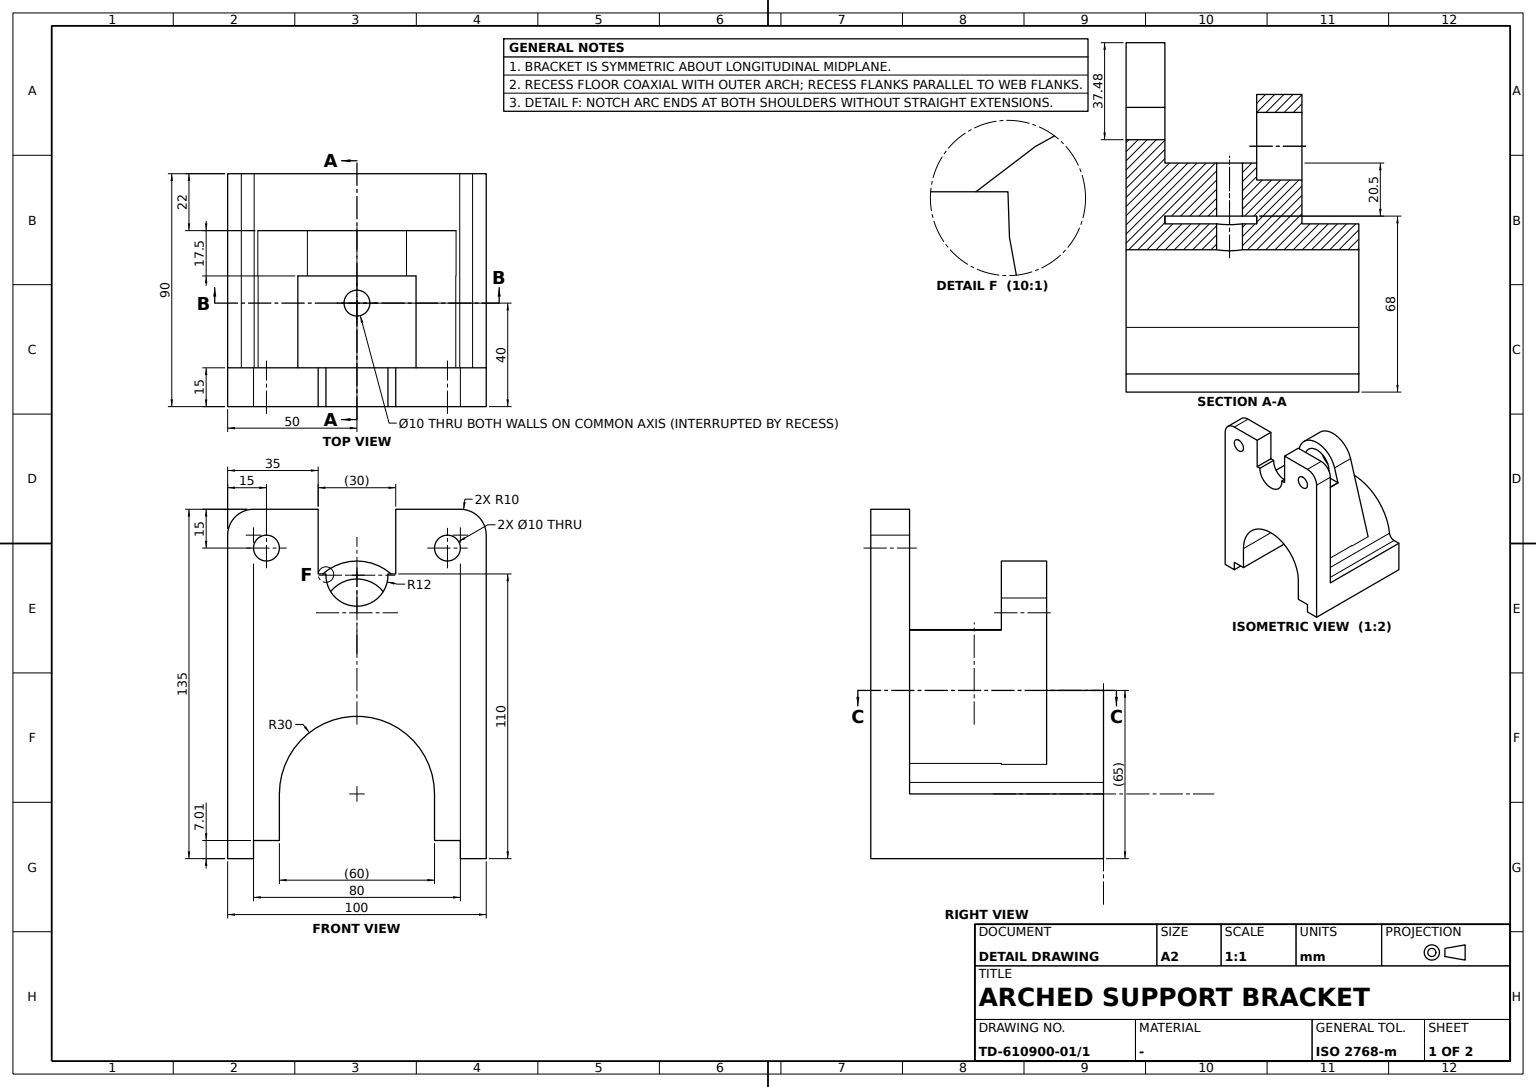
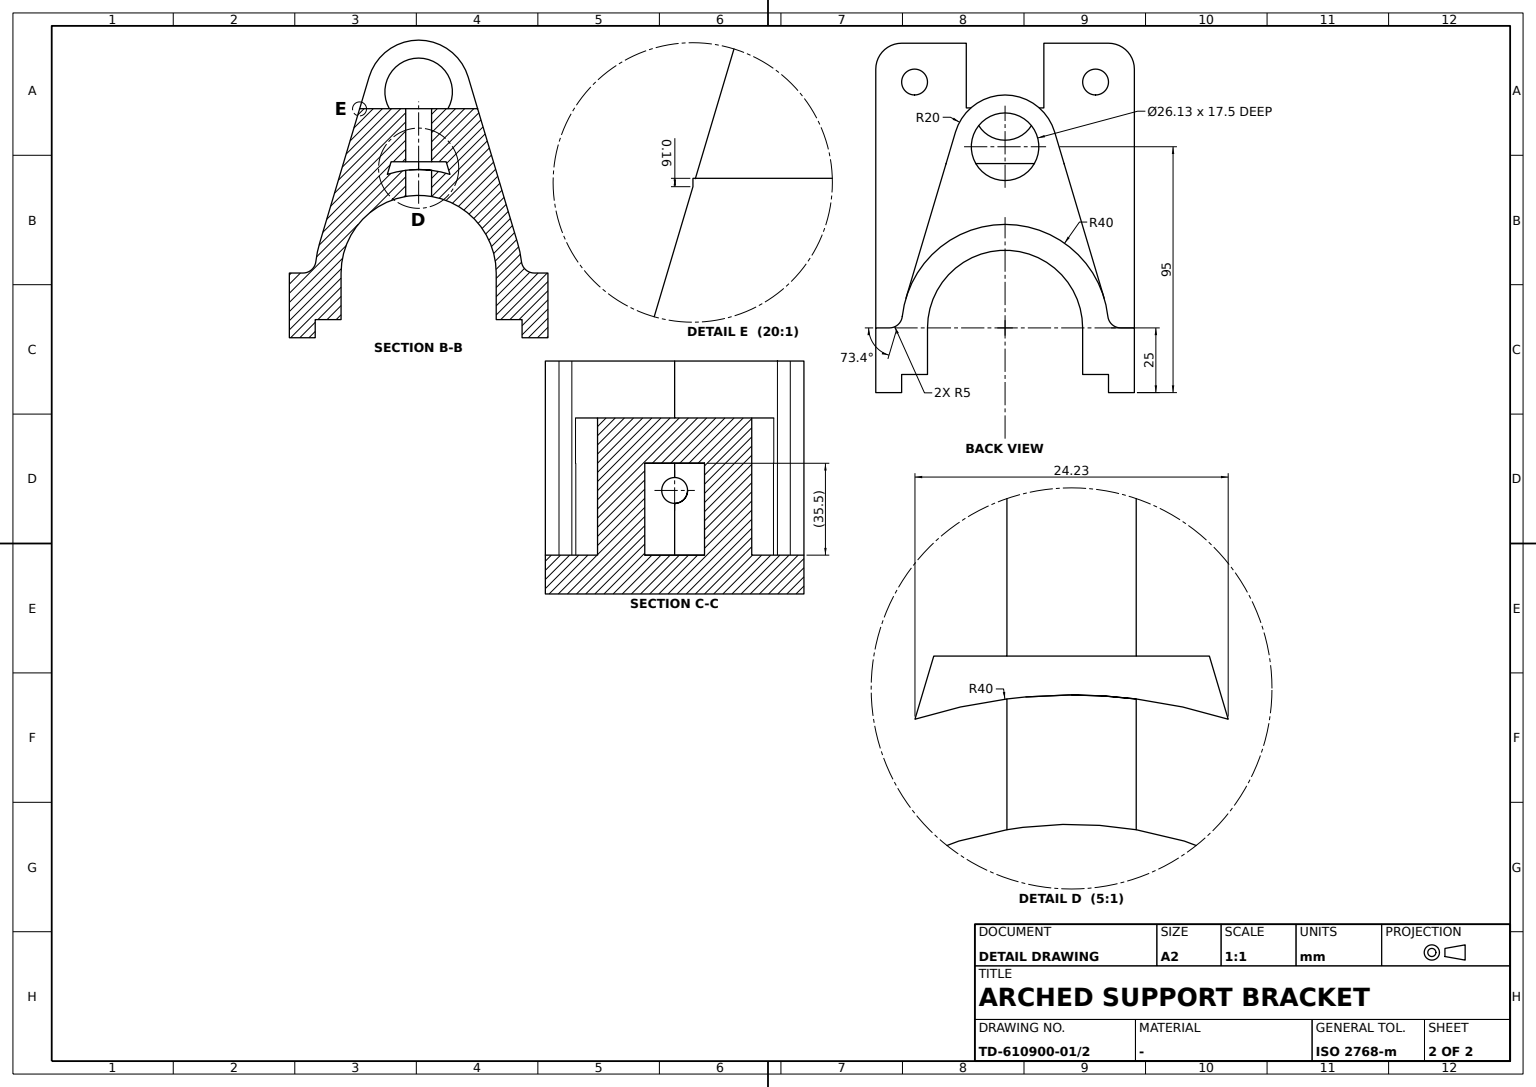
CATIA V5 part; units mm, degrees
sketch "Sketch1" plane through (0, 0, 0) normal (0, 0, 1) x (1, 0, 0)
  line L0 (-50, 45) -> (50, 45)
  line L1 (50, 45) -> (50, -45)
  line L2 (50, -45) -> (-50, -45)
  line L3 (-50, -45) -> (-50, 45)
  dimension "length L1" = 90
  dimension "length L2" = 100
  constraint horizontal L0 x-axis
  constraint horizontal L2 x-axis
  constraint vertical L1 y-axis
  constraint vertical L3 y-axis
  constraint symmetry L3 L1 y-axis
  constraint symmetry L0 L2 x-axis
extrude "Pad1" add sketch "Sketch1" along normal blind 25
sketch "Sketch2" plane through (0, 45, 0) normal (0, 1, 0) x (-1, 0, 0)
  arc A0 (40, 25) -> (-40, 25) centre (0, 25) ccw
  point P0 (0, 25)
  line L0 (-50, 25) -> (50, 25) construction
  line L1 (-50, 25) -> (50, 25) construction
  line L2 (-40, 25) -> (40, 25)
  point P1 (-40, 25)
  point P2 (40, 25)
  dimension "radius A0" = 40
  constraint coincidence P0 y-axis
  constraint coincidence P0 L0
  constraint coincidence L1 P1
  constraint coincidence L1 P2
extrude "Pad2" add sketch "Sketch2" against normal blind 90
sketch "Sketch3" plane through (0, 45, 0) normal (0, 1, 0) x (-1, 0, 0)
  arc A0 (30, 25) -> (-30, 25) centre (0, 25) ccw
  point P0 (0, 25)
  arc A1 (40, 25) -> (-40, 25) centre (0, 25) ccw construction
  line L0 (-30, 25) -> (30, 25)
  dimension "radius A0" = 30
  constraint coincidence P0 y-axis
  constraint concentricity A1 A0
  constraint horizontal L0 x-axis
extrude "Pocket1" cut sketch "Sketch3" against normal blind 90
sketch "Sketch4" plane through (0, 45, 0) normal (0, 1, 0) x (-1, 0, 0)
  line L0 (-30, 1.8224) -> (-30, 11.8224)
  line L1 (-30, 11.8224) -> (30, 11.8224)
  line L2 (30, 11.8224) -> (30, 1.8224)
  line L3 (30, 1.8224) -> (-30, 1.8224)
  dimension "length L0" = 10
  dimension "length L3" = 60
  constraint vertical L0 y-axis
  constraint vertical L2 y-axis
  constraint horizontal L1 x-axis
  constraint horizontal L3 x-axis
  constraint symmetry L0 L2 y-axis
extrude "Pocket2" cut sketch "Sketch4" against normal blind 90
sketch "Sketch5" plane through (0, 45, 0) normal (0, 1, 0) x (-1, 0, 0)
  line L0 (-30, 25) -> (30, 25)
  line L1 (30, 25) -> (30, 11.8224)
  line L2 (30, 11.8224) -> (-30, 11.8224)
  line L3 (-30, 11.8224) -> (-30, 25)
  point P0 (30, 11.8224)
  point P1 (-30, 11.8224)
  line L4 (30, 11.8224) -> (-30, 11.8224) construction
  line L5 (-30, 25) -> (30, 25) construction
  point P2 (30, 11.8224)
  point P3 (-30, 11.8224)
  constraint horizontal L0 x-axis
  constraint horizontal L2 x-axis
  constraint vertical L1 y-axis
  constraint vertical L3 y-axis
  constraint coincidence L2 L4
  constraint coincidence L0 L5
  constraint coincidence P0 P2
  constraint coincidence P3 P1
extrude "Pocket3" cut sketch "Sketch5" against normal blind 90
sketch "Sketch6" plane through (0, 45, 0) normal (0, 1, 0) x (-1, 0, 0)
  point P0 (-40, 0)
  line L0 (-40, 0) -> (-40, 7.006)
  line L1 (-40, 7.006) -> (40, 7.006)
  line L2 (40, 7.006) -> (40, 0)
  point P1 (40, 0)
  line L3 (40, 0) -> (-40, 0)
  point P2 (-40, 0)
  dimension "length L3" = 80
  constraint vertical L0 y-axis
  constraint vertical L2 y-axis
  constraint horizontal L1 x-axis
  constraint horizontal L3 x-axis
  constraint coincidence P1 x-axis
  constraint coincidence P2 L0
  constraint coincidence P0 P2
  constraint symmetry L0 L2 y-axis
extrude "Pocket4" cut sketch "Sketch6" against normal blind 90
sketch "Sketch7" plane through (0, -45, 0) normal (0, -1, 0) x (1, 0, 0)
  point P0 (-50, 25)
  line L0 (-50, 25) -> (50, 25)
  line L1 (50, 25) -> (50, 135)
  line L2 (50, 135) -> (-50, 135)
  line L3 (-50, 135) -> (-50, 25)
  point P1 (50, 25)
  point P2 (-50, 25)
  point P3 (50, 25)
  dimension "length L1" = 110
  constraint horizontal L0 x-axis
  constraint horizontal L2 x-axis
  constraint vertical L1 y-axis
  constraint vertical L3 y-axis
  constraint coincidence P2 P0
  constraint coincidence P1 P3
extrude "Pad3" add sketch "Sketch7" against normal blind 15
sketch "Sketch8" plane through (0, -30, 0) normal (0, 1, 0) x (-1, 0, 0)
  line L0 (-15, 135) -> (15, 135)
  line L1 (15, 135) -> (15, 110)
  line L2 (15, 110) -> (-15, 110)
  line L3 (-15, 110) -> (-15, 135)
  line L4 (-50, 135) -> (50, 135) construction
  dimension "length L0" = 30
  dimension "length L1" = 25
  constraint horizontal L0 x-axis
  constraint horizontal L2 x-axis
  constraint vertical L1 y-axis
  constraint vertical L3 y-axis
  constraint coincidence L0 L4
  constraint symmetry L3 L1 y-axis
extrude "Pocket5" cut sketch "Sketch8" against normal blind 15
sketch "Sketch9" plane through (0, -30, 0) normal (0, 1, 0) x (-1, 0, 0)
  circle A0 centre (0, 109.5177) radius 12
  point P0 (0, 109.5177)
  dimension "radius A0" = 12
  constraint coincidence P0 y-axis
extrude "Pocket6" cut sketch "Sketch9" against normal blind 15
sketch "Sketch10" plane through (0, -30, 0) normal (0, 1, 0) x (-1, 0, 0)
  circle A0 centre (-35, 120) radius 5
  point P0 (-35, 120)
  circle A1 centre (35, 120) radius 5
  point P1 (35, 120)
  line L0 (-50, 135) -> (50, 135) construction
  line L1 (-50, 135) -> (50, 135) construction
  dimension "radius A1" = 5
  dimension "radius A0" = 5
  dimension "distance y axis P1" = 35
  dimension "distance P0 y axis" = 35
  dimension "distance L0 P1" = 15
  dimension "distance P0 L1" = 15
extrude "Pocket7" cut sketch "Sketch10" against normal blind 15
fillet "Fillet1" radius 10 2 edges at (50, -37.5, 135) (-50, -37.5, 135)
ref_plane "Plane1" through (0, 23, 0) normal (0, 1, 0) x (1, 0, 0)
sketch "Sketch11" plane through (0, 23, 0) normal (0, -1, 0) x (1, 0, 0)
  arc A0 (40, 25) -> (-40, 25) centre (0, 25) ccw construction
  arc A1 (38.3326, 36.4286) -> (-38.3326, 36.4286) centre (0, 25) ccw
  point P0 (0, 95)
  arc A2 (19.1663, 100.7143) -> (-19.1663, 100.7143) centre (0, 95) ccw
  line L0 (38.3326, 36.4286) -> (19.1663, 100.7143)
  line L1 (-19.1663, 100.7143) -> (-38.3326, 36.4286)
  point P1 (38.3326, 36.4286)
  point P2 (-38.3326, 36.4286)
  dimension "distance x axis P0" = 95
  dimension "radius A2" = 20
  constraint coincidence P0 y-axis
  constraint coincidence A0 P1
  constraint coincidence A0 P2
  constraint tangency A2 L0
  constraint tangency A2 L1
  constraint tangency A0 L1
  constraint tangency L0 A0
extrude "Pad4" add sketch "Sketch11" along normal blind 17.5
sketch "Sketch12" plane through (0, 23, 0) normal (0, 1, 0) x (-1, 0, 0)
  circle A0 centre (0, 95) radius 13.0625
  point P0 (0, 95)
  arc A1 (19.1663, 100.7143) -> (-19.1663, 100.7143) centre (0, 95) ccw construction
  constraint coincidence P0 y-axis
  constraint concentricity A1 A0
extrude "Pocket8" cut sketch "Sketch12" against normal blind 17.5
fillet "Fillet2" radius 5 2 edges at (40, 7.5, 25) (-40, 7.5, 25)
ref_plane "Plane2" through (0, 0, 68) normal (0, 0, 1) x (1, 0, 0)
sketch "Sketch13" plane through (45.1777, 0, 13.4694) normal (0.9583, 0, 0.2857) x (0, 1, 0)
  line L0 (-30.0717, 78.1257) -> (-30.0717, 24.3451)
  line L1 (-30.0717, 24.3451) -> (22.4266, 24.3451)
  line L2 (22.4266, 24.3451) -> (22.4266, 78.1257)
  line L3 (22.4266, 78.1257) -> (-30.0717, 78.1257)
  constraint vertical L0 y-axis
  constraint vertical L2 y-axis
  constraint horizontal L1 x-axis
  constraint horizontal L3 x-axis
extrude "Pad5" add sketch "Sketch13" against normal blind 17.5
mirror "Mirror1" about plane through (0, 0, 0) normal (1, 0, 0)
sketch "Sketch14" plane through (0, 0, 68) normal (0, 0, 1) x (1, 0, 0)
  line L0 (-22.8561, 5.5) -> (22.8561, 5.5)
  line L1 (22.8561, 5.5) -> (22.8561, -30)
  line L2 (22.8561, -30) -> (-22.8561, -30)
  line L3 (-22.8561, -30) -> (-22.8561, 5.5)
  line L4 (-22.8561, 5.5) -> (-22.8561, -30) construction
  line L5 (22.8561, 22.4266) -> (22.8561, -30.0717) construction
  line L6 (12, -30) -> (-12, -30) construction
  line L7 (19.1663, 5.5) -> (-19.1663, 5.5) construction
  constraint horizontal L0 x-axis
  constraint horizontal L2 x-axis
  constraint vertical L1 y-axis
  constraint vertical L3 y-axis
  constraint coincidence L3 L4
  constraint coincidence L1 L5
  constraint coincidence L2 L6
  constraint coincidence L7 L0
extrude "Pad6" add sketch "Sketch14" along normal blind 20.5
sketch "Sketch15" plane through (0, 0, 88.5) normal (0, 0, 1) x (1, 0, 0)
  circle A0 centre (0, -5) radius 5
  point P0 (0, -5)
  line L0 (12, -30) -> (-12, -30) construction
  dimension "radius A0" = 5
  dimension "distance L0 P0" = 25
  constraint coincidence P0 y-axis
extrude "Pocket9" cut sketch "Sketch15" against normal through all
sketch "Sketch16" plane through (0, 45, 0) normal (0, 1, 0) x (-1, 0, 0)
  arc A0 (30, 25) -> (-30, 25) centre (0, 25) ccw
extrude "Pocket10" cut sketch "Sketch16" against normal through all material side at (0, 45, 54.95)
